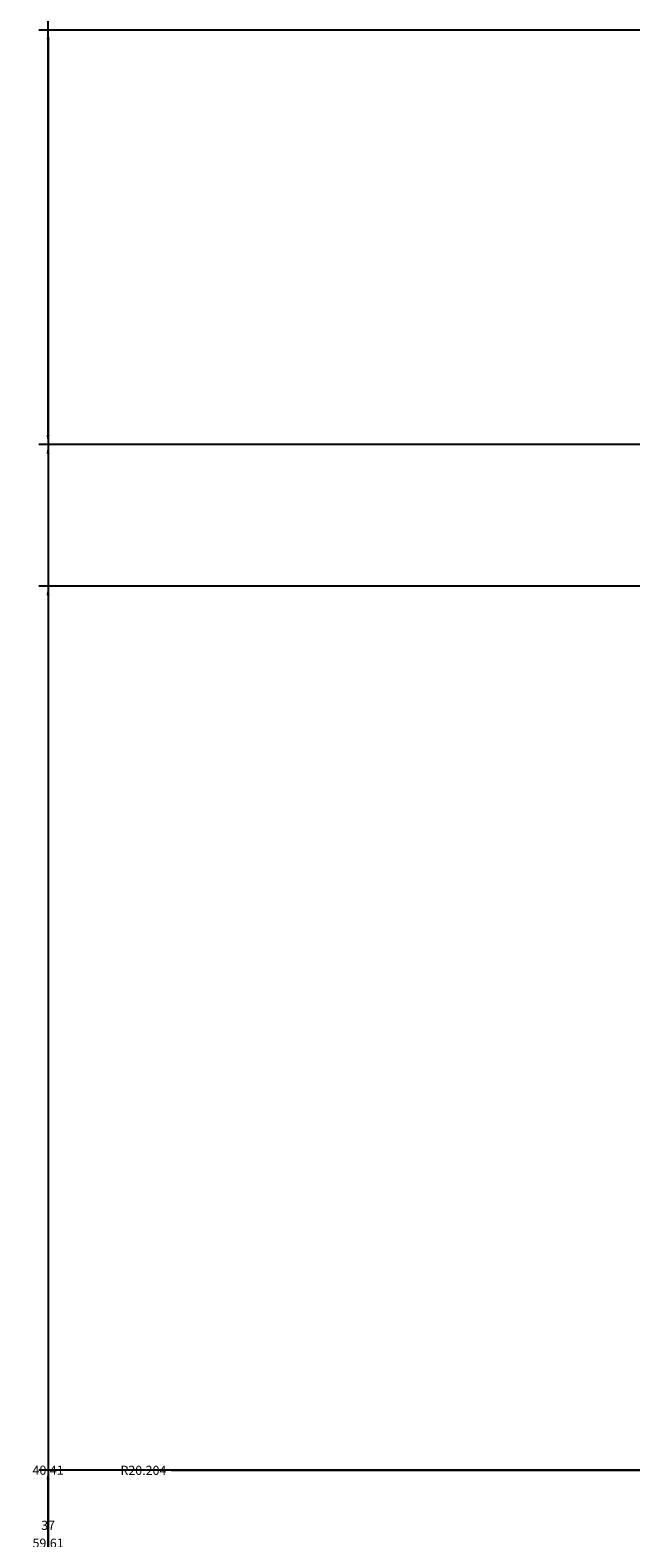
# Model space of a CAD drawing. Units: inches. Extents: x -12 to 334, y -10 to 186.
# Tile 6 of 77: x -12 to 0, y 79 to 109. Entities that reach past the tile are written whole.
import ezdxf

# ---------------------------------------------------------------- set-up
doc = ezdxf.new("R2010")
doc.units = ezdxf.units.IN
doc.header["$MEASUREMENT"] = 0
doc.layers.add('M-DIMS', color=2, linetype='Continuous', lineweight=18)
doc.styles.get("Standard").update_dxf_attribs({"font": 'arial.ttf'})
doc.dimstyles.get("Standard").update_dxf_attribs({"dimtxt": 0.18, "dimasz": 0.18, "dimexe": 0.18, "dimexo": 0.0625, "dimgap": 0.09, "dimtad": 0, "dimtih": 1, "dimtoh": 1, "dimdec": 4, "dimzin": 0, "dimdsep": 46, "dimtxsty": 'Standard', "dimcen": 0.09, "dimadec": 0, "dimazin": 0, "dimtfac": 1, "dimtdec": 4, "dimtofl": 0, "dimtmove": 0, "dimatfit": 3, "dimfxl": 1, "dimtolj": 1, "dimtzin": 0, "dimarcsym": 0})

# ---------------------------------------------------------------- blocks, each defined once
blk = doc.blocks.new('*D7')
at = {"layer": 'Defpoints', "color": 0, "transparency": 16777216}
for p in [(-11.174, 100.896), (23.581, 100.896), (23.581, 60.487)]:
    blk.add_point(p, dxfattribs=at)
at = {"layer": 'M-DIMS', "color": 0, "lineweight": -2, "transparency": 16777216}
for p, q in [((23.518, 100.896), (-11.354, 100.896)), ((-11.174, 100.716), (-11.174, 80.873)), ((-11.174, 60.667), (-11.174, 80.51)), ((23.518, 60.487), (-11.354, 60.487))]:
    blk.add_line(p, q, dxfattribs=at)
at = {"layer": 'M-DIMS', "color": 0, "transparency": 16777216}
for points in [[(-11.204, 100.716), (-11.144, 100.716), (-11.174, 100.896)], [(-11.204, 60.667), (-11.144, 60.667), (-11.174, 60.487)]]:
    blk.add_solid(points, dxfattribs=at)
at = {"layer": 'M-DIMS', "color": 0, "transparency": 16777216, "insert": (-11.174, 80.692), "char_height": 0.18, "attachment_point": 5}
blk.add_mtext('\\A1;40.41', dxfattribs=at)
blk = doc.blocks.new('*D8')
at = {"layer": 'Defpoints', "color": 0, "transparency": 16777216}
for p in [(-11.174, 127.708), (32.1, 127.708), (23.581, 100.896)]:
    blk.add_point(p, dxfattribs=at)
at = {"layer": 'M-DIMS', "color": 0, "lineweight": -2, "transparency": 16777216}
for p, q in [((32.038, 127.708), (-11.354, 127.708)), ((-11.174, 127.528), (-11.174, 114.484)), ((-11.174, 101.076), (-11.174, 114.12)), ((23.518, 100.896), (-11.354, 100.896))]:
    blk.add_line(p, q, dxfattribs=at)
at = {"layer": 'M-DIMS', "color": 0, "transparency": 16777216}
for points in [[(-11.204, 127.528), (-11.144, 127.528), (-11.174, 127.708)], [(-11.204, 101.076), (-11.144, 101.076), (-11.174, 100.896)]]:
    blk.add_solid(points, dxfattribs=at)
at = {"layer": 'M-DIMS', "color": 0, "transparency": 16777216, "insert": (-11.174, 114.302), "char_height": 0.18, "attachment_point": 5}
blk.add_mtext('\\A1;26.81', dxfattribs=at)
blk = doc.blocks.new('*D14')
at = {"layer": 'Defpoints', "color": 0, "transparency": 16777216}
for p in [(63.5, 109.058), (-11.174, 49.45), (64.207, 49.45)]:
    blk.add_point(p, dxfattribs=at)
at = {"layer": 'M-DIMS', "color": 0, "lineweight": -2, "transparency": 16777216}
for p, q in [((63.438, 109.058), (-11.354, 109.058)), ((-11.174, 108.878), (-11.174, 79.436)), ((-11.174, 49.63), (-11.174, 79.072)), ((64.144, 49.45), (-11.354, 49.45))]:
    blk.add_line(p, q, dxfattribs=at)
at = {"layer": 'M-DIMS', "color": 0, "transparency": 16777216}
for points in [[(-11.204, 108.878), (-11.144, 108.878), (-11.174, 109.058)], [(-11.204, 49.63), (-11.144, 49.63), (-11.174, 49.45)]]:
    blk.add_solid(points, dxfattribs=at)
at = {"layer": 'M-DIMS', "color": 0, "transparency": 16777216, "insert": (-11.174, 79.254), "char_height": 0.18, "attachment_point": 5}
blk.add_mtext('\\A1;59.61', dxfattribs=at)
blk = doc.blocks.new('*D35')
at = {"layer": 'Defpoints', "color": 0, "transparency": 16777216}
for p in [(216.428, 98.108), (-11.174, 61.105), (216.428, 61.105)]:
    blk.add_point(p, dxfattribs=at)
at = {"layer": 'M-DIMS', "color": 0, "lineweight": -2, "transparency": 16777216}
for p, q in [((216.365, 98.108), (-11.354, 98.108)), ((-11.174, 97.928), (-11.174, 79.788)), ((-11.174, 61.285), (-11.174, 79.424)), ((216.365, 61.105), (-11.354, 61.105))]:
    blk.add_line(p, q, dxfattribs=at)
at = {"layer": 'M-DIMS', "color": 0, "transparency": 16777216}
for points in [[(-11.204, 97.928), (-11.144, 97.928), (-11.174, 98.108)], [(-11.204, 61.285), (-11.144, 61.285), (-11.174, 61.105)]]:
    blk.add_solid(points, dxfattribs=at)
at = {"layer": 'M-DIMS', "color": 0, "transparency": 16777216, "insert": (-11.174, 79.606), "char_height": 0.18, "attachment_point": 5}
blk.add_mtext('\\A1;37', dxfattribs=at)
blk = doc.blocks.new('*D39')
at = {"layer": 'Defpoints', "color": 0, "transparency": 16777216}
for p in [(279.726, 80.692), (-11.174, 45.854), (269.381, 45.854)]:
    blk.add_point(p, dxfattribs=at)
at = {"layer": 'M-DIMS', "color": 0, "lineweight": -2, "transparency": 16777216}
for p, q in [((279.664, 80.692), (-11.354, 80.692)), ((-11.174, 80.512), (-11.174, 63.455)), ((-11.174, 46.034), (-11.174, 63.091)), ((269.318, 45.854), (-11.354, 45.854))]:
    blk.add_line(p, q, dxfattribs=at)
at = {"layer": 'M-DIMS', "color": 0, "transparency": 16777216}
for points in [[(-11.204, 80.512), (-11.144, 80.512), (-11.174, 80.692)], [(-11.204, 46.034), (-11.144, 46.034), (-11.174, 45.854)]]:
    blk.add_solid(points, dxfattribs=at)
at = {"layer": 'M-DIMS', "color": 0, "transparency": 16777216, "insert": (-11.174, 63.273), "char_height": 0.18, "attachment_point": 5}
blk.add_mtext('\\A1;34.84', dxfattribs=at)
blk = doc.blocks.new('*D42')
at = {"layer": 'Defpoints', "color": 0, "transparency": 16777216}
for p in [(3.376, 80.69), (23.581, 80.692)]:
    blk.add_point(p, dxfattribs=at)
at = {"layer": 'M-DIMS', "color": 0, "lineweight": -2, "transparency": 16777216}
for p, q in [((23.581, 80.602), (23.581, 80.782)), ((-8.746, 80.689), (3.196, 80.69)), ((23.491, 80.692), (23.671, 80.692))]:
    blk.add_line(p, q, dxfattribs=at)
at = {"layer": 'M-DIMS', "color": 0, "transparency": 16777216}
blk.add_solid([(3.196, 80.72), (3.196, 80.66), (3.376, 80.69)], dxfattribs=at)
at = {"layer": 'M-DIMS', "color": 0, "transparency": 16777216, "insert": (-9.296, 80.689), "char_height": 0.18, "attachment_point": 5}
blk.add_mtext('\\A1;R20.204', dxfattribs=at)

msp = doc.modelspace()

# ---------------------------------------------------------------- dimensions: what is measured, and where the dimension line sits
at = {"layer": 'M-DIMS'}
for base, p1, p2, override, picture, middle in [((-11.1736, 127.7078), (23.5807, 100.8958), (32.1002, 127.7078), {"dimdec": 2, "dimlfac": 1, "dimrnd": 0, "dimzin": 0, "dimdsep": 46, "dimlunit": 2}, '*D8', (-11.1735, 114.3018)), ((-11.1736, 49.4497), (63.5, 109.0583), (64.2068, 49.4497), {"dimdec": 2, "dimlfac": 1, "dimrnd": 0, "dimzin": 0, "dimdsep": 46, "dimlunit": 2}, '*D14', (-11.1735, 79.254)), ((-11.1736, 100.8958), (23.5807, 60.4872), (23.5807, 100.8958), {"dimdec": 2, "dimlfac": 1, "dimrnd": 0, "dimzin": 0, "dimdsep": 46, "dimlunit": 2}, '*D7', (-11.1735, 80.6915)), ((-11.1736, 61.1045), (216.4278, 98.1081), (216.4278, 61.1045), {"dimdec": 0, "dimlfac": 1, "dimrnd": 0, "dimzin": 0, "dimdsep": 46, "dimlunit": 2}, '*D35', (-11.1735, 79.6063)), ((-11.1736, 45.8541), (279.7263, 80.6915), (269.3808, 45.8541), {"dimdec": 2, "dimlfac": 1, "dimrnd": 0, "dimzin": 0, "dimdsep": 46, "dimlunit": 2}, '*D39', (-11.1735, 63.2728))]:
    dim = msp.add_linear_dim(base=base, p1=p1, p2=p2, angle=90, dimstyle='Standard', override=override, dxfattribs=at)
    dim.commit()
    dim.dimension.update_dxf_attribs({"geometry": picture, "text_midpoint": middle})
dim = msp.add_radius_dim(center=(23.5807, 80.6915), mpoint=(3.3764, 80.69), dimstyle='Standard', override={"dimdec": 3, "dimlfac": 1, "dimrnd": 0, "dimzin": 0, "dimdsep": 46, "dimlunit": 2}, dxfattribs=at)
dim.commit()
dim.dimension.update_dxf_attribs({"geometry": '*D42', "text_midpoint": (-8.7461, 80.6891), "dimtype": 164})

doc.saveas('drawing.dxf')
